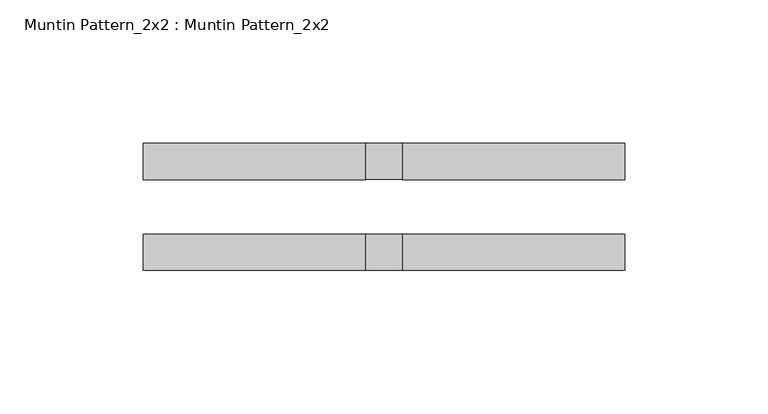
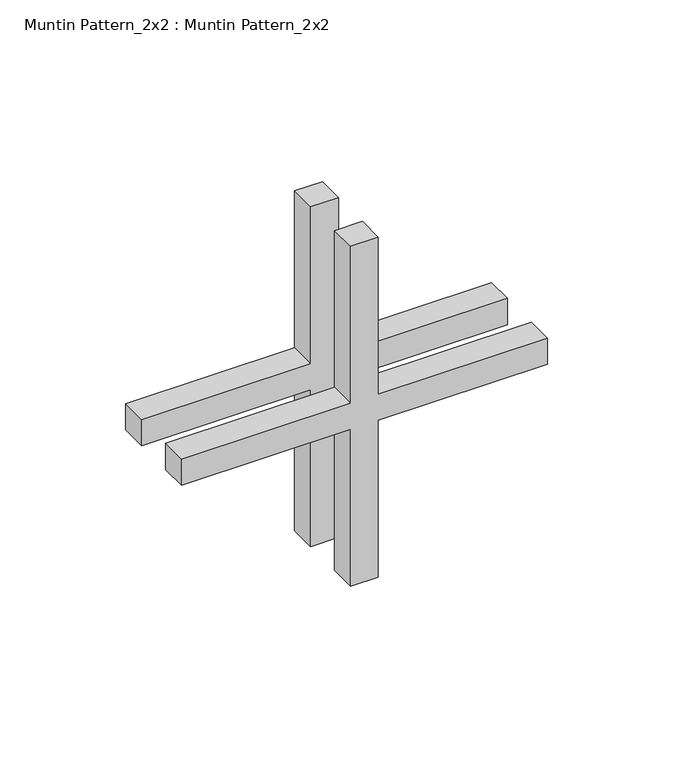
"""IFC4 building model written with IfcOpenShell, lengths in millimetres: proxy geometry, Muntin Pattern_2x2 : Muntin Pattern_2x2."""

from ifc_helpers import new_model, si_unit, frame, origin, place, context, project, spatial, polyline, outline, extrude, source, transform, mapped, element, save


def muntin_pattern_2x2_muntin_pattern_2x2_4939cdd6(model_context):
    return source(origin(), model_context, "Body", "SweptSolid", [
        extrude(outline(polyline([(88.9, -6.35), (88.9, -84.1375), (76.2, -84.1375), (76.2, -6.35), (0.0, -6.35), (0.0, 6.35), (76.2, 6.35), (76.2, 84.1375), (88.9, 84.1375), (88.9, 6.35), (165.1, 6.35), (165.1, -6.35), (88.9, -6.35)])), frame((0.0, 9.525, 0.0), z_axis=(0.0, 1.0, 0.0), x_axis=(0.0, 0.0, 1.0)), (0.0, 0.0, 1.0), 12.7),
        extrude(outline(polyline([(88.9, -6.35), (88.9, -84.1375), (76.2, -84.1375), (76.2, -6.35), (0.0, -6.35), (0.0, 6.35), (76.2, 6.35), (76.2, 84.1375), (88.9, 84.1375), (88.9, 6.35), (165.1, 6.35), (165.1, -6.35), (88.9, -6.35)])), frame((0.0, -22.225, 0.0), z_axis=(0.0, 1.0, 0.0), x_axis=(0.0, 0.0, 1.0)), (0.0, 0.0, 1.0), 12.7),
    ])


if __name__ == "__main__":
    model = new_model("IFC4")
    model_context = context("Model", 3, world=origin())
    ifc_project = project(units=[si_unit("LENGTHUNIT", "METRE", prefix="MILLI")], contexts=[model_context])
    site = spatial("IfcSite", under=ifc_project)
    building = spatial("IfcBuilding", under=site)
    placement = place(None, origin())
    muntin_pattern_2x2_muntin_pattern_2x2_shape = muntin_pattern_2x2_muntin_pattern_2x2_4939cdd6(model_context)
    element("IfcBuildingElementProxy", 1, Name="Muntin Pattern_2x2 : Muntin Pattern_2x2", ObjectType="Muntin Pattern_2x2 : Muntin Pattern_2x2", at=placement, inside=building, context=model_context, shape_type="MappedRepresentation", body=[
        mapped(muntin_pattern_2x2_muntin_pattern_2x2_shape, transform((0.0, 0.0, 0.0), x_axis=(1.0, 0.0, 0.0), y_axis=(0.0, 1.0, 0.0), z_axis=(0.0, 0.0, 1.0))),
    ])
    save(model, "model.ifc")

# Revit data of these elements
# Type "Muntin Pattern_2x2 : Muntin Pattern_2x2"
#   Width [instance default] = 4' - 0"
#   Thickness = 0' - 0 1/2"
#   Height [instance default] = 4' - 0"
#   Distance = 0' - 0 3/4"
#   Interior Material [instance default] = none
#   Exterior Material [instance default] = none
#   Default Elevation = 0
# Element 1 (IfcBuildingElementProxy, "Muntin Pattern_2x2 : Muntin Pattern_2x2")
#   Width = 0' - 6 5/8"
#   Height = 0' - 6 1/2"
#   Interior Material = Wood - Stained
#   Exterior Material = Clad - White
#   Materials on its faces: "Clad - White", "Wood - Stained"
# Materials
#   "Clad - White": class "Wood", colour RGB 242 242 238, transparency 0, Cost = 0
#   "Wood - Stained": class "Wood", colour RGB 224 178 126, transparency 0, Cost = 0
